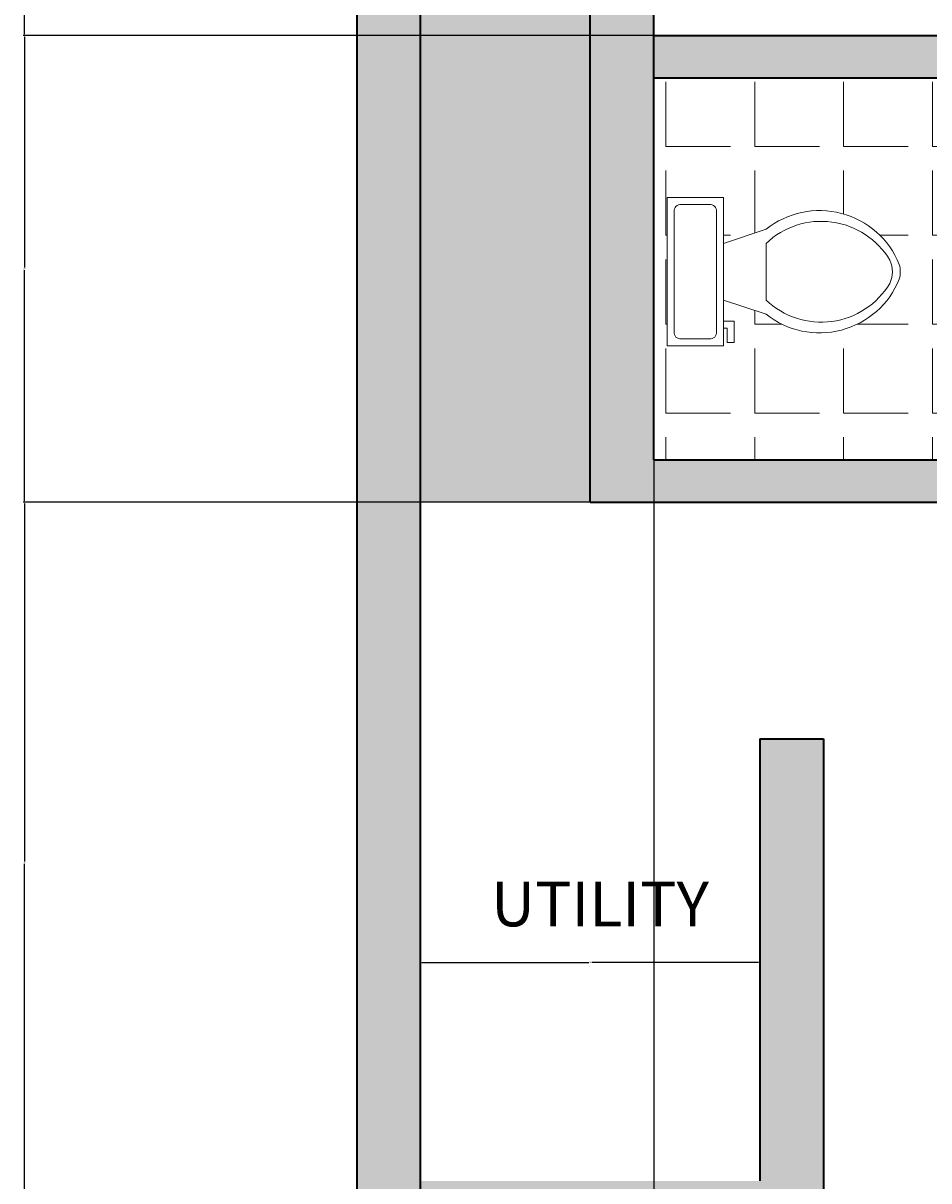
# Model space of a CAD drawing. Units: inches. Extents: x 2549 to 3108, y 1683 to 2362.
# Tile 6 of 30: x 2549 to 2678, y 1979 to 2142. Entities that reach past the tile are written whole.
import ezdxf

# ---------------------------------------------------------------- set-up
doc = ezdxf.new("R2010")
doc.units = ezdxf.units.IN
for name, color, linetype, lineweight in [('A-ANNO-DIMS', 2, 'Continuous', 18), ('A-AREA-IDEN', 7, 'Continuous', 18), ('A-FLOR', 7, 'Continuous', 25), ('A-FLOR-FIXT', 9, 'Continuous', 18), ('A-FLOR-PATT', 8, 'Continuous', 13), ('A-FURN-PATT', 9, 'Continuous', 13), ('A-WALL', 7, 'Continuous', 35), ('A-WALL-PATT', 89, 'Continuous', 13), ('C-PROP', 7, 'Continuous', 35)]:
    doc.layers.add(name, color=color, linetype=linetype, lineweight=lineweight)
for name, color, linetype, lineweight, true_color in [('C-PKNG-VEHI-PATT', 251, 'Continuous', 13, 0x636466), ('C-PROP-PATT', 252, 'Continuous', 13, 0x939598), ('C-PVMT-PATT', 9, 'Continuous', 13, 0xc7c8ca)]:
    doc.layers.add(name, color=color, linetype=linetype, lineweight=lineweight, true_color=true_color)
doc.styles.get("Standard").update_dxf_attribs({"font": 'arial.ttf'})
doc.dimstyles.get("Standard").update_dxf_attribs({"dimtxt": 0.18, "dimasz": 0.18, "dimexe": 0.18, "dimexo": 0.0625, "dimgap": 0.09, "dimtad": 0, "dimtih": 1, "dimtoh": 1, "dimdec": 4, "dimzin": 0, "dimdsep": 46, "dimtxsty": 'Standard', "dimcen": 0.09, "dimadec": 0, "dimazin": 0, "dimtfac": 1, "dimtdec": 4, "dimtofl": 0, "dimtmove": 0, "dimatfit": 3, "dimfxl": 1, "dimtolj": 1, "dimtzin": 0, "dimarcsym": 0})

# ---------------------------------------------------------------- blocks, each defined once
blk = doc.blocks.new('*U3')
for p, q in [((9.5, -6), (9.5, -2)), ((-8, -8.5), (-8, -8)), ((-7, -8), (-7, -9.5)), ((-4, -8), (-6, -14)), ((4, -8), (6, -14)), ((-10, -8.5), (-8, -8.5)), ((-10, -9.5), (-10, -8.5)), ((-7, -9.5), (-10, -9.5)), ((4, -14), (-4, -14))]:
    blk.add_line(p, q)
blk.add_lwpolyline([(10.5, -8), (10.5, 0), (-10.5, 0), (-10.5, -8)], close=True)
for points in [[(8.5, -1), (-8.5, -1)], [(-9.5, -2), (-9.5, -6)], [(-8.5, -7), (8.5, -7)]]:
    blk.add_lwpolyline(points)
for centre, radius, start, end in [((-8.62, -1.88), 0.884, 81.8699, 188.1301), ((8.62, -1.88), 0.884, 351.8699, 98.1301), ((-8.62, -6.12), 0.884, 171.8699, 278.1301), ((8.62, -6.12), 0.884, 261.8699, 8.1301), ((3.52, -21.58), 12.17, 141.4691, 247.9714), ((4.2, -21.82), 11.33, 136.3677, 238.9468), ((-3.52, -21.58), 12.17, 292.0284, 38.5307), ((-4.2, -21.82), 11.33, 301.053, 43.6321), ((0, -27.88), 4, 245.7318, 294.2682), ((0, -29), 4, 254.8605, 285.1395)]:
    blk.add_arc(centre, radius, start, end)
blk = doc.blocks.new('*D32')
at = {"layer": 'A-ANNO-DIMS', "color": 0, "lineweight": -2, "transparency": 16777216}
for p, q in [((2629.58, 2281.52), (2549.42, 2281.52)), ((2549.6, 2281.34), (2549.6, 2211.2)), ((2549.6, 2140.7), (2549.6, 2210.84)), ((2638.58, 2140.52), (2549.42, 2140.52))]:
    blk.add_line(p, q, dxfattribs=at)
at = {"layer": 'A-ANNO-DIMS', "color": 0, "transparency": 16777216}
for points in [[(2549.57, 2281.34), (2549.63, 2281.34), (2549.6, 2281.52)], [(2549.57, 2140.7), (2549.63, 2140.7), (2549.6, 2140.52)]]:
    blk.add_solid(points, dxfattribs=at)
at = {"layer": 'Defpoints', "color": 0, "transparency": 16777216}
for p in [(2549.6, 2281.52), (2629.64, 2281.52), (2638.64, 2140.52)]:
    blk.add_point(p, dxfattribs=at)
at = {"layer": 'A-ANNO-DIMS', "color": 0, "transparency": 16777216, "insert": (2549.6, 2211.02), "char_height": 0.18, "attachment_point": 5}
blk.add_mtext('\\A1;141', dxfattribs=at)
blk = doc.blocks.new('*D33')
at = {"layer": 'A-ANNO-DIMS', "color": 0, "lineweight": -2, "transparency": 16777216}
for p, q in [((2638.58, 2140.52), (2549.42, 2140.52)), ((2549.6, 2140.34), (2549.6, 2107.71)), ((2549.6, 2074.7), (2549.6, 2107.34)), ((2629.58, 2074.52), (2549.42, 2074.52))]:
    blk.add_line(p, q, dxfattribs=at)
at = {"layer": 'A-ANNO-DIMS', "color": 0, "transparency": 16777216}
for points in [[(2549.57, 2140.34), (2549.63, 2140.34), (2549.6, 2140.52)], [(2549.57, 2074.7), (2549.63, 2074.7), (2549.6, 2074.52)]]:
    blk.add_solid(points, dxfattribs=at)
at = {"layer": 'Defpoints', "color": 0, "transparency": 16777216}
for p in [(2549.6, 2140.52), (2638.64, 2140.52), (2629.64, 2074.52)]:
    blk.add_point(p, dxfattribs=at)
at = {"layer": 'A-ANNO-DIMS', "color": 0, "transparency": 16777216, "insert": (2549.6, 2107.52), "char_height": 0.18, "attachment_point": 5}
blk.add_mtext('\\A1;66', dxfattribs=at)
blk = doc.blocks.new('*D34')
at = {"layer": 'A-ANNO-DIMS', "color": 0, "lineweight": -2, "transparency": 16777216}
for p, q in [((2629.58, 2074.52), (2549.42, 2074.52)), ((2549.6, 2074.34), (2549.6, 2023.71)), ((2549.6, 1972.7), (2549.6, 2023.34)), ((2638.58, 1972.52), (2549.42, 1972.52))]:
    blk.add_line(p, q, dxfattribs=at)
at = {"layer": 'A-ANNO-DIMS', "color": 0, "transparency": 16777216}
for points in [[(2549.57, 2074.34), (2549.63, 2074.34), (2549.6, 2074.52)], [(2549.57, 1972.7), (2549.63, 1972.7), (2549.6, 1972.52)]]:
    blk.add_solid(points, dxfattribs=at)
at = {"layer": 'Defpoints', "color": 0, "transparency": 16777216}
for p in [(2549.6, 2074.52), (2629.64, 2074.52), (2638.64, 1972.52)]:
    blk.add_point(p, dxfattribs=at)
at = {"layer": 'A-ANNO-DIMS', "color": 0, "transparency": 16777216, "insert": (2549.6, 2023.52), "char_height": 0.18, "attachment_point": 5}
blk.add_mtext('\\A1;102', dxfattribs=at)
blk = doc.blocks.new('*D42')
at = {"layer": 'A-ANNO-DIMS', "color": 0, "lineweight": -2, "transparency": 16777216}
for p, q in [((2638.64, 2080.46), (2638.64, 1683.44)), ((2728.64, 2080.46), (2728.64, 1683.44)), ((2638.82, 1683.62), (2683.42, 1683.62)), ((2728.46, 1683.62), (2683.86, 1683.62))]:
    blk.add_line(p, q, dxfattribs=at)
at = {"layer": 'A-ANNO-DIMS', "color": 0, "transparency": 16777216}
for points in [[(2638.82, 1683.65), (2638.82, 1683.59), (2638.64, 1683.62)], [(2728.46, 1683.65), (2728.46, 1683.59), (2728.64, 1683.62)]]:
    blk.add_solid(points, dxfattribs=at)
at = {"layer": 'Defpoints', "color": 0, "transparency": 16777216}
for p in [(2638.64, 2080.52), (2728.64, 2080.52), (2728.64, 1683.62)]:
    blk.add_point(p, dxfattribs=at)
at = {"layer": 'A-ANNO-DIMS', "color": 0, "transparency": 16777216, "insert": (2683.64, 1683.62), "char_height": 0.18, "attachment_point": 5}
blk.add_mtext('\\A1;90', dxfattribs=at)
blk = doc.blocks.new('*D44')
at = {"layer": 'A-ANNO-DIMS', "color": 0, "lineweight": -2, "transparency": 16777216}
for p, q in [((2662.64, 2040.99), (2662.64, 1683.44)), ((2806.64, 2016.13), (2806.64, 1683.44)), ((2662.82, 1683.62), (2734.36, 1683.62)), ((2806.46, 1683.62), (2734.92, 1683.62))]:
    blk.add_line(p, q, dxfattribs=at)
at = {"layer": 'A-ANNO-DIMS', "color": 0, "transparency": 16777216}
for points in [[(2662.82, 1683.65), (2662.82, 1683.59), (2662.64, 1683.62)], [(2806.46, 1683.65), (2806.46, 1683.59), (2806.64, 1683.62)]]:
    blk.add_solid(points, dxfattribs=at)
at = {"layer": 'Defpoints', "color": 0, "transparency": 16777216}
for p in [(2662.64, 2041.06), (2806.64, 2016.19), (2806.64, 1683.62)]:
    blk.add_point(p, dxfattribs=at)
at = {"layer": 'A-ANNO-DIMS', "color": 0, "transparency": 16777216, "insert": (2734.64, 1683.62), "char_height": 0.18, "attachment_point": 5}
blk.add_mtext('\\A1;144', dxfattribs=at)
blk = doc.blocks.new('*D45')
at = {"layer": 'A-ANNO-DIMS', "color": 0, "lineweight": -2, "transparency": 16777216}
for p, q in [((2605.64, 1978.59), (2605.64, 2009.6)), ((2605.82, 2009.42), (2629.42, 2009.42)), ((2653.46, 2009.42), (2629.87, 2009.42)), ((2653.64, 1978.59), (2653.64, 2009.6))]:
    blk.add_line(p, q, dxfattribs=at)
at = {"layer": 'A-ANNO-DIMS', "color": 0, "transparency": 16777216}
for points in [[(2605.82, 2009.45), (2605.82, 2009.39), (2605.64, 2009.42)], [(2653.46, 2009.45), (2653.46, 2009.39), (2653.64, 2009.42)]]:
    blk.add_solid(points, dxfattribs=at)
at = {"layer": 'Defpoints', "color": 0, "transparency": 16777216}
for p in [(2653.64, 2009.42), (2605.64, 1978.52), (2653.64, 1978.52)]:
    blk.add_point(p, dxfattribs=at)
at = {"layer": 'A-ANNO-DIMS', "color": 0, "transparency": 16777216, "insert": (2629.64, 2009.42), "char_height": 0.18, "attachment_point": 5}
blk.add_mtext('\\A1;48', dxfattribs=at)

msp = doc.modelspace()

# ---------------------------------------------------------------- hatches: boundary and pattern name
at = {"layer": 'A-FLOR-PATT', "transparency": 33554567}
h = msp.add_hatch(dxfattribs=at)
h.set_pattern_fill('ANGLE', color=256, scale=1.8)
h.set_pattern_definition([(0, (0, 0), (0, 12.573), [9.144, -3.429]), (90, (0, 0), (-12.573, 8e-16), [9.144, -3.429])])
h.paths.add_polyline_path([(2806.6427, 2134.5237), (2785.7177, 2134.5237), (2747.213, 2134.5237), (2638.6427, 2134.5237), (2638.6427, 2080.5237), (2728.6427, 2080.5237), (2728.6427, 2109.4935), (2734.6427, 2109.4935), (2734.6427, 2080.5237), (2806.6427, 2080.5237)])
h.paths.add_polyline_path([(2673.3659, 2106.0669, -0.50131678), (2654.5049, 2101.1116), (2648.5048, 2103.1116), (2648.5048, 2100.1116), (2650.0048, 2100.1116), (2650.0048, 2097.1116), (2649.0048, 2097.1116), (2649.0048, 2099.1116), (2648.5048, 2099.1116), (2648.5048, 2096.6116), (2640.5048, 2096.6116), (2640.5048, 2117.6116), (2648.5048, 2117.6116), (2648.5048, 2111.1116), (2654.5047, 2113.1116, -0.50132349), (2673.3659, 2108.1563, -0.13289091)], flags=16)
h.paths.add_polyline_path([(2672.0278, 2105.4676, -0.48007965), (2654.5048, 2103.1117), (2654.5048, 2111.1116, -0.4800795), (2672.0278, 2108.7557, -0.21500378)], flags=0)
h.paths.add_polyline_path([(2647.5048, 2115.6116), (2647.5048, 2098.6116, -0.50000012), (2646.5048, 2097.6116), (2642.5048, 2097.6116, -0.50000012), (2641.5048, 2098.6116), (2641.5048, 2115.6116, -0.50000012), (2642.5048, 2116.6116), (2646.5048, 2116.6116, -0.50000012)], flags=0)
h.paths.add_polyline_path([(2748.8496, 2101.6383), (2798.148, 2101.6383), (2798.148, 2111.4248), (2748.8496, 2111.4248)], flags=24)
h.paths.add_polyline_path([(2685.2081, 2101.489), (2719.3253, 2101.489), (2719.3253, 2111.2819), (2685.2081, 2111.2819)], flags=24)
at = {"layer": 'A-FURN-PATT', "transparency": 33554567}
h = msp.add_hatch(color=256, dxfattribs=at)
h.dxf.hatch_style = 1
h.paths.add_polyline_path([(2708.7147, 2271.6737), (2675.2813, 2271.6737), (2675.2813, 2262.0404), (2708.7147, 2262.0404)])
h.paths.add_polyline_path([(2980.8246, 2271.6737), (2947.3913, 2271.6737), (2947.3913, 2262.0404), (2980.8246, 2262.0404)])
h.paths.add_polyline_path([(2748.8496, 2101.6383), (2798.148, 2101.6383), (2798.148, 2111.4248), (2748.8496, 2111.4248)], flags=9)
h.paths.add_polyline_path([(2685.2081, 2101.489), (2719.3253, 2101.489), (2719.3253, 2111.2819), (2685.2081, 2111.2819)], flags=9)
h.paths.add_polyline_path([(2814.6852, 1907.1328), (2847.8384, 1907.1328), (2847.8384, 1916.9258), (2814.6852, 1916.9258)], flags=9)
h.paths.add_polyline_path([(2814.3906, 1835.5864), (2848.0172, 1835.5864), (2848.0172, 1845.3794), (2814.3906, 1845.3794)], flags=9)
h.paths.add_polyline_path([(2800.5245, 1759.1674), (2853.7435, 1759.1674), (2853.7435, 1768.954), (2800.5245, 1768.954)], flags=9)
h.paths.add_polyline_path([(2972.4611, 1807.3305), (3015.3943, 1807.3305), (3015.3943, 1817.117), (2972.4611, 1817.117)], flags=9)
h.paths.add_polyline_path([(2902.3327, 1888.6731), (2937.9131, 1888.6731), (2937.9131, 1898.4661), (2902.3327, 1898.4661)], flags=9)
h.paths.add_polyline_path([(2712.1779, 1878.9039), (2754.1257, 1878.9039), (2754.1257, 1888.6904), (2712.1779, 1888.6904)], flags=9)
h.paths.add_polyline_path([(2614.0056, 2012.812), (2650.0251, 2012.812), (2650.0251, 2022.4371), (2614.0056, 2022.4371)], flags=9)
h.paths.add_polyline_path([(2713.3129, 2003.1645), (2747.4237, 2003.1645), (2747.4237, 2012.951), (2713.3129, 2012.951)], flags=9)
h.paths.add_polyline_path([(2950.1379, 2001.6934), (2982.2992, 2001.6934), (2982.2992, 2011.48), (2950.1379, 2011.48)], flags=9)
h.paths.add_polyline_path([(2940.864, 2238.5537), (2997.5066, 2238.5537), (2997.5066, 2248.3466), (2940.864, 2248.3466)], flags=9)
h.paths.add_polyline_path([(2821.5457, 2202.8348), (2855.663, 2202.8348), (2855.663, 2212.6278), (2821.5457, 2212.6278)], flags=9)
h.paths.add_polyline_path([(2661.8026, 2238.6249), (2718.4451, 2238.6249), (2718.4451, 2248.4179), (2661.8026, 2248.4179)], flags=9)
h = msp.add_hatch(color=256, dxfattribs=at)
h.dxf.hatch_style = 1
h.paths.add_polyline_path([(2906.5064, 1905.2148), (2905.2584, 1904.3827), (2907.0611, 1900.7772), (2908.3092, 1901.6092)])
h.paths.add_polyline_path([(2936.522, 1914.8044), (2935.2739, 1915.6364), (2932.6391, 1912.5856), (2933.8871, 1911.7535)])
h.paths.add_polyline_path([(2950.2508, 1905.6518), (2949.0027, 1906.4839), (2947.1999, 1902.8783), (2948.448, 1902.0463)])
h.paths.add_polyline_path([(2958.5713, 1918.1326), (2956.9072, 1919.242), (2952.4696, 1908.98, 1.38742744), (2954.9657, 1907.3159)])
h.paths.add_polyline_path([(2945.2585, 1927.0078), (2943.5944, 1928.1172), (2934.9965, 1920.6287, 1.38742744), (2937.4927, 1918.9646)])
h.paths.add_polyline_path([(2748.8496, 2101.6383), (2798.148, 2101.6383), (2798.148, 2111.4248), (2748.8496, 2111.4248)], flags=9)
h.paths.add_polyline_path([(2685.2081, 2101.489), (2719.3253, 2101.489), (2719.3253, 2111.2819), (2685.2081, 2111.2819)], flags=9)
h.paths.add_polyline_path([(2814.6852, 1907.1328), (2847.8384, 1907.1328), (2847.8384, 1916.9258), (2814.6852, 1916.9258)], flags=9)
h.paths.add_polyline_path([(2814.3906, 1835.5864), (2848.0172, 1835.5864), (2848.0172, 1845.3794), (2814.3906, 1845.3794)], flags=9)
h.paths.add_polyline_path([(2800.5245, 1759.1674), (2853.7435, 1759.1674), (2853.7435, 1768.954), (2800.5245, 1768.954)], flags=9)
h.paths.add_polyline_path([(2972.4611, 1807.3305), (3015.3943, 1807.3305), (3015.3943, 1817.117), (2972.4611, 1817.117)], flags=9)
h.paths.add_polyline_path([(2902.3327, 1888.6731), (2937.9131, 1888.6731), (2937.9131, 1898.4661), (2902.3327, 1898.4661)], flags=9)
h.paths.add_polyline_path([(2712.1779, 1878.9039), (2754.1257, 1878.9039), (2754.1257, 1888.6904), (2712.1779, 1888.6904)], flags=9)
h.paths.add_polyline_path([(2614.0056, 2012.812), (2650.0251, 2012.812), (2650.0251, 2022.4371), (2614.0056, 2022.4371)], flags=9)
h.paths.add_polyline_path([(2713.3129, 2003.1645), (2747.4237, 2003.1645), (2747.4237, 2012.951), (2713.3129, 2012.951)], flags=9)
h.paths.add_polyline_path([(2950.1379, 2001.6934), (2982.2992, 2001.6934), (2982.2992, 2011.48), (2950.1379, 2011.48)], flags=9)
h.paths.add_polyline_path([(2940.864, 2238.5537), (2997.5066, 2238.5537), (2997.5066, 2248.3466), (2940.864, 2248.3466)], flags=9)
h.paths.add_polyline_path([(2821.5457, 2202.8348), (2855.663, 2202.8348), (2855.663, 2212.6278), (2821.5457, 2212.6278)], flags=9)
h.paths.add_polyline_path([(2661.8026, 2238.6249), (2718.4451, 2238.6249), (2718.4451, 2248.4179), (2661.8026, 2248.4179)], flags=9)
at = {"layer": 'A-WALL-PATT'}
h = msp.add_hatch(color=256, dxfattribs=at)
h.dxf.hatch_style = 1
h.paths.add_polyline_path([(2638.6427, 2272.5237), (3034.6427, 2272.5237), (3034.6427, 1936.5237), (3043.6427, 1936.5237), (3043.6427, 2281.5237), (2629.6427, 2281.5237), (2629.6427, 2074.5237), (2812.6427, 2074.5237), (2812.6427, 2140.5237), (2785.7177, 2140.5237), (2785.7177, 2134.5237), (2806.6427, 2134.5237), (2806.6427, 2080.5237), (2638.6427, 2080.5237)])
h.paths.add_polyline_path([(2638.6427, 1972.5237), (2662.6427, 1972.5237), (2662.6427, 2041.0557), (2653.6427, 2041.0557), (2653.6427, 1978.5237), (2629.6427, 1978.5237), (2629.6427, 1795.5237), (2662.6427, 1795.5237), (2881.6427, 1795.5237), (2881.6427, 1936.5237), (2965.9351, 1936.5237), (2965.9351, 1974.5439), (2959.9351, 1974.5439), (2959.9351, 1945.5237), (2881.6427, 1945.5237), (2872.6427, 1945.5237), (2872.6427, 1804.5237), (2662.6427, 1804.5237), (2638.6427, 1804.5237)])
h = msp.add_hatch(color=256, dxfattribs=at)
h.dxf.hatch_style = 1
h.paths.add_polyline_path([(2747.213, 2140.5237), (2638.6427, 2140.5237), (2638.6427, 2134.5237), (2747.213, 2134.5237)])
h.paths.add_polyline_path([(2734.6427, 2109.4935), (2728.6427, 2109.4935), (2728.6427, 2080.5237), (2734.6427, 2080.5237)])
h.paths.add_polyline_path([(2812.6427, 2074.5237), (2806.6427, 2074.5237), (2806.6427, 2016.1911), (2812.6427, 2016.1911)])
h.paths.add_polyline_path([(2812.6427, 1945.5237), (2806.6427, 1945.5237), (2806.6427, 1885.5237), (2872.6427, 1885.5237), (2872.6427, 1891.5237), (2812.6427, 1891.5237)])
h.paths.add_polyline_path([(2812.6427, 1855.9859), (2806.6427, 1855.9859), (2806.6427, 1804.5237), (2812.6427, 1804.5237)])
at = {"layer": 'C-PKNG-VEHI-PATT'}
h = msp.add_hatch(color=256, dxfattribs=at)
h.dxf.hatch_style = 1
edge = h.paths.add_edge_path()
edge.add_ellipse((2935.7258, 1791.964), major_axis=(-50.66, 0), ratio=0.84230387, start_angle=248.165046, end_angle=265.722579)
edge.add_line((2938.911, 1834.5507), (2925.8653, 1834.5507))
edge.add_ellipse((2929.0505, 1791.964), major_axis=(50.66, 0), ratio=0.84230387, start_angle=94.277421, end_angle=111.834954)
edge.add_line((2912.8508, 1832.3947), (2914.2044, 1822.2495))
edge.add_ellipse((2930.6538, 1783.1023), major_axis=(-49.3014, 0), ratio=0.84230387, start_angle=-85.12993, end_angle=-67.208085, ccw=False)
edge.add_line((2927.1247, 1824.5225), (2937.6516, 1824.5225))
edge.add_ellipse((2934.1225, 1783.1023), major_axis=(49.3014, 0), ratio=0.84230387, start_angle=67.208085, end_angle=85.12993, ccw=False)
edge.add_line((2950.5719, 1822.2495), (2951.9255, 1832.3947))
edge = h.paths.add_edge_path()
edge.add_ellipse((2903.4793, 1857.3351), major_axis=(-34.7979, 0), ratio=0.84230387, start_angle=180, end_angle=209.43857)
edge.add_ellipse((2961.297, 1857.3351), major_axis=(34.7979, 0), ratio=0.84230387, start_angle=150.56143, end_angle=180)
edge.add_line((2926.4991, 1857.3351), (2926.4991, 1843.7609))
edge.add_ellipse((2924.1251, 1844.3143), major_axis=(-0.2209, 3.9278), ratio=0.60383358, start_angle=89.002014, end_angle=253.657408, ccw=False)
edge.add_line((2921.7512, 1844.2222), (2921.7512, 1853.3975))
edge.add_line((2921.7512, 1853.3975), (2925.269, 1855.8484))
edge.add_ellipse((2925.4782, 1855.4931), major_axis=(0.4584, 0), ratio=0.84230387, start_angle=90, end_angle=134.480211, ccw=False)
edge.add_line((2925.4782, 1855.8792), (2926.4991, 1855.8792))
edge.add_line((2926.4991, 1855.8792), (2926.4991, 1857.3351))
edge.add_ellipse((2961.297, 1857.3351), major_axis=(34.7979, 0), ratio=0.84230387, start_angle=150.56143, end_angle=180, ccw=False)
edge.add_line((2932.3882, 1873.6501), (2932.3882, 1875.7801))
edge.add_ellipse((2932.3882, 1875.3939), major_axis=(0.4584, 0), ratio=0.84230387, start_angle=90, end_angle=127.93313)
edge.add_line((2932.1366, 1875.7167), (2928.5915, 1873.7564))
edge.add_ellipse((2899.9271, 2002.4692), major_axis=(155.4756, 0), ratio=0.84230387, start_angle=-80.743434, end_angle=-77.445067, ccw=False)
edge.add_ellipse((2949.4402, 1715.2151), major_axis=(-189.1422, 0), ratio=0.84230387, start_angle=-79.790461, end_angle=-77.555373)
edge.add_ellipse((3300.3614, 1852.5642), major_axis=(-386.1662, 0), ratio=0.84230387, start_angle=-2.863715, end_angle=2.198541)
edge.add_ellipse((2929.0505, 1792.5159), major_axis=(-55.6192, 0), ratio=0.84230387, start_angle=-85.917589, end_angle=-72.280047, ccw=False)
edge.add_line((2925.7129, 1839.2798), (2939.0634, 1839.2798))
edge.add_ellipse((2935.7258, 1792.5159), major_axis=(55.6192, 0), ratio=0.84230387, start_angle=72.280047, end_angle=85.917589, ccw=False)
edge.add_ellipse((2564.4149, 1852.5642), major_axis=(-386.1662, 0), ratio=0.84230387, start_angle=177.801459, end_angle=182.863715)
edge.add_ellipse((2915.3361, 1715.2151), major_axis=(189.1422, 0), ratio=0.84230387, start_angle=77.555373, end_angle=79.790461)
edge.add_ellipse((2964.8492, 2002.4692), major_axis=(-155.4756, 0), ratio=0.84230387, start_angle=77.445067, end_angle=80.743434, ccw=False)
edge.add_line((2936.1848, 1873.7564), (2932.6397, 1875.7167))
edge.add_ellipse((2932.3882, 1875.3939), major_axis=(0.4584, 0), ratio=0.84230387, start_angle=52.06687, end_angle=90)
edge.add_line((2932.3882, 1875.7801), (2932.3882, 1873.6501))
edge.add_ellipse((2903.4793, 1857.3351), major_axis=(-34.7979, 0), ratio=0.84230387, start_angle=180, end_angle=209.43857, ccw=False)
edge.add_line((2938.2772, 1857.3351), (2938.2772, 1855.8792))
edge.add_line((2938.2772, 1855.8792), (2939.4059, 1855.8792))
edge.add_ellipse((2939.2981, 1855.4931), major_axis=(-0.4584, 0), ratio=0.84230387, start_angle=225.519789, end_angle=270, ccw=False)
edge.add_line((2939.5903, 1855.7906), (2943.0251, 1853.3975))
edge.add_line((2943.0251, 1853.3975), (2943.0251, 1844.2222))
edge.add_ellipse((2940.6512, 1844.3143), major_axis=(0.2209, 3.9278), ratio=0.60383358, start_angle=106.342592, end_angle=270.997986, ccw=False)
edge.add_line((2938.2772, 1843.7609), (2938.2772, 1857.3351))
edge = h.paths.add_edge_path()
edge.add_ellipse((2932.3882, 1865.1973), major_axis=(91.081, 0), ratio=0.84230387, start_angle=256.401865, end_angle=283.598135, ccw=False)
edge.add_line((2914.2044, 1790.0239), (2914.2044, 1778.3622))
edge.add_ellipse((2932.3882, 1853.5356), major_axis=(91.081, 0), ratio=0.84230387, start_angle=256.401865, end_angle=283.598135)
edge.add_line((2950.5719, 1778.3622), (2950.5719, 1790.0239))
edge = h.paths.add_edge_path()
edge.add_ellipse((2948.7383, 1772.3145), major_axis=(1.8336, 0), ratio=0.84230387, start_angle=0, end_angle=90)
edge.add_line((2948.7383, 1773.859), (2916.038, 1773.859))
edge.add_ellipse((2916.038, 1772.3145), major_axis=(1.8336, 0), ratio=0.84230387, start_angle=90, end_angle=180)
edge.add_line((2914.2044, 1772.3145), (2914.2044, 1760.2558))
edge.add_line((2914.2044, 1760.2558), (2950.5719, 1760.2558))
edge.add_line((2950.5719, 1760.2558), (2950.5719, 1772.3145))
h.paths.add_polyline_path([(2748.8496, 2101.6383), (2798.148, 2101.6383), (2798.148, 2111.4248), (2748.8496, 2111.4248)], flags=9)
h.paths.add_polyline_path([(2685.2081, 2101.489), (2719.3253, 2101.489), (2719.3253, 2111.2819), (2685.2081, 2111.2819)], flags=9)
h.paths.add_polyline_path([(2814.6852, 1907.1328), (2847.8384, 1907.1328), (2847.8384, 1916.9258), (2814.6852, 1916.9258)], flags=9)
h.paths.add_polyline_path([(2814.3906, 1835.5864), (2848.0172, 1835.5864), (2848.0172, 1845.3794), (2814.3906, 1845.3794)], flags=9)
h.paths.add_polyline_path([(2800.5245, 1759.1674), (2853.7435, 1759.1674), (2853.7435, 1768.954), (2800.5245, 1768.954)], flags=9)
h.paths.add_polyline_path([(2972.4611, 1807.3305), (3015.3943, 1807.3305), (3015.3943, 1817.117), (2972.4611, 1817.117)], flags=9)
h.paths.add_polyline_path([(2902.3327, 1888.6731), (2937.9131, 1888.6731), (2937.9131, 1898.4661), (2902.3327, 1898.4661)], flags=9)
h.paths.add_polyline_path([(2712.1779, 1878.9039), (2754.1257, 1878.9039), (2754.1257, 1888.6904), (2712.1779, 1888.6904)], flags=9)
h.paths.add_polyline_path([(2614.0056, 2012.812), (2650.0251, 2012.812), (2650.0251, 2022.4371), (2614.0056, 2022.4371)], flags=9)
h.paths.add_polyline_path([(2713.3129, 2003.1645), (2747.4237, 2003.1645), (2747.4237, 2012.951), (2713.3129, 2012.951)], flags=9)
h.paths.add_polyline_path([(2950.1379, 2001.6934), (2982.2992, 2001.6934), (2982.2992, 2011.48), (2950.1379, 2011.48)], flags=9)
h.paths.add_polyline_path([(2940.864, 2238.5537), (2997.5066, 2238.5537), (2997.5066, 2248.3466), (2940.864, 2248.3466)], flags=9)
h.paths.add_polyline_path([(2821.5457, 2202.8348), (2855.663, 2202.8348), (2855.663, 2212.6278), (2821.5457, 2212.6278)], flags=9)
h.paths.add_polyline_path([(2661.8026, 2238.6249), (2718.4451, 2238.6249), (2718.4451, 2248.4179), (2661.8026, 2248.4179)], flags=9)
at = {"layer": 'C-PROP-PATT'}
h = msp.add_hatch(color=256, dxfattribs=at)
h.dxf.hatch_style = 1
h.paths.add_polyline_path([(3076.6427, 2314.5237), (2596.6427, 2314.5237), (2596.6427, 1714.5237), (2881.84, 1714.5237), (2881.84, 1723.5237), (2605.6427, 1723.5237), (2605.6427, 2305.5237), (3067.6427, 2305.5237), (3067.6427, 1723.5237), (3067.6427, 1714.5237), (3076.6427, 1714.5237)])
at = {"layer": 'C-PVMT-PATT'}
h = msp.add_hatch(color=256, dxfattribs=at)
h.dxf.hatch_style = 1
h.paths.add_polyline_path([(3067.6427, 2305.5237), (2605.6427, 2305.5237), (2605.6427, 2074.5237), (2629.6427, 2074.5237), (2629.6427, 2281.5237), (3043.6427, 2281.5237), (3043.6427, 1885.5237), (3043.6427, 1872.8745), (3031.1672, 1872.8745), (3031.1672, 1862.5731), (2995.8054, 1862.5731), (2995.8054, 1872.8745), (2983.1752, 1872.8745), (2983.1752, 1885.5237), (2881.6427, 1885.5237), (2881.6427, 1795.5237), (2751.0977, 1795.5237), (2751.0977, 1761.5237), (2786.1577, 1761.5237), (2786.1577, 1723.5237), (2881.84, 1723.5237), (2881.84, 1714.5237), (3067.6427, 1714.5237), (3067.6427, 1723.5237)])
edge = h.paths.add_edge_path(flags=16)
edge.add_ellipse((2949.4402, 1710.9683), major_axis=(-194.1014, 0), ratio=0.84230387, start_angle=-77.874034, end_angle=-76.219471, ccw=False)
edge.add_ellipse((2949.4402, 1715.2151), major_axis=(-189.1422, 0), ratio=0.84230387, start_angle=-79.790461, end_angle=-77.555373, ccw=False)
edge.add_ellipse((2899.9271, 2002.4692), major_axis=(155.4756, 0), ratio=0.84230387, start_angle=-80.743434, end_angle=-77.445067)
edge.add_line((2928.5915, 1873.7564), (2932.3882, 1875.8558))
edge.add_line((2932.3882, 1875.8558), (2936.1848, 1873.7564))
edge.add_ellipse((2964.8492, 2002.4692), major_axis=(-155.4756, 0), ratio=0.84230387, start_angle=77.445067, end_angle=80.743434)
edge.add_ellipse((2915.3361, 1715.2151), major_axis=(189.1422, 0), ratio=0.84230387, start_angle=77.555373, end_angle=79.790461, ccw=False)
edge.add_ellipse((2915.3361, 1710.9683), major_axis=(-194.1014, 0), ratio=0.84230387, start_angle=256.219471, end_angle=257.874034, ccw=False)
edge.add_ellipse((2628.2871, 1850.2612), major_axis=(-327.2532, 0), ratio=0.84230387, start_angle=182.17995, end_angle=183.650428, ccw=False)
edge.add_ellipse((2955.5637, 1861.9334), major_axis=(-0.9168, 0), ratio=0.84230387, start_angle=180, end_angle=270, ccw=False)
edge.add_line((2956.4805, 1862.3857), (2956.4805, 1846.4866))
edge.add_ellipse((2955.5637, 1846.939), major_axis=(-0.9168, 0), ratio=0.84230387, start_angle=90, end_angle=180, ccw=False)
edge.add_ellipse((-3607.0606, 1835.832), major_axis=(-6562.6242, 0), ratio=0.84230387, start_angle=179.61613322, end_angle=180.09022909, ccw=False)
edge.add_ellipse((2955.5637, 1791.0926), major_axis=(0.9168, 0), ratio=0.84230387, start_angle=0, end_angle=90, ccw=False)
edge.add_line((2956.4805, 1791.545), (2956.4805, 1775.6459))
edge.add_ellipse((2955.5637, 1776.0982), major_axis=(0.9168, 0), ratio=0.84230387, start_angle=270, end_angle=360, ccw=False)
edge.add_ellipse((-3607.0606, 1835.832), major_axis=(-6562.6242, 0), ratio=0.84230387, start_angle=179.3813568, end_angle=179.47172853, ccw=False)
edge.add_ellipse((2954.5907, 1763.8768), major_axis=(-1.3752, 0), ratio=0.84230387, start_angle=179.371763, end_angle=248.464757, ccw=False)
edge.add_ellipse((-3607.519, 1835.832), major_axis=(-6564.0409, 0), ratio=0.842303863, start_angle=179.35344594, end_angle=179.37176282, ccw=False)
edge.add_ellipse((2952.6829, 1761.8002), major_axis=(3.2503, 0), ratio=0.84230387, start_angle=-90, end_angle=-0.646554, ccw=False)
edge.add_line((2952.6829, 1759.0625), (2912.0934, 1759.0625))
edge.add_ellipse((2912.0934, 1761.8002), major_axis=(3.2503, 0), ratio=0.84230387, start_angle=180.646554, end_angle=270, ccw=False)
edge.add_ellipse((9472.2953, 1835.832), major_axis=(-6564.0409, 0), ratio=0.842303871, start_angle=0.62823722, end_angle=0.6465541, ccw=False)
edge.add_ellipse((2910.1856, 1763.8768), major_axis=(1.3752, 0), ratio=0.84230387, start_angle=111.535244, end_angle=180.628237, ccw=False)
edge.add_ellipse((9471.8369, 1835.832), major_axis=(-6562.6242, 0), ratio=0.84230387, start_angle=0.52827147, end_angle=0.6465541, ccw=False)
edge.add_ellipse((2909.2126, 1776.0982), major_axis=(-0.9168, 0), ratio=0.84230387, start_angle=0, end_angle=90, ccw=False)
edge.add_line((2908.2958, 1775.6459), (2908.2958, 1791.545))
edge.add_ellipse((2909.2126, 1791.0926), major_axis=(-0.9168, 0), ratio=0.84230387, start_angle=-90, end_angle=0, ccw=False)
edge.add_ellipse((9471.8369, 1835.832), major_axis=(-6562.6242, 0), ratio=0.84230387, start_angle=-0.09022909, end_angle=0.38386678, ccw=False)
edge.add_ellipse((2909.2126, 1846.939), major_axis=(-0.9168, 0), ratio=0.84230387, start_angle=0, end_angle=90, ccw=False)
edge.add_line((2908.2958, 1846.4866), (2908.2958, 1862.3857))
edge.add_ellipse((2909.2126, 1861.9334), major_axis=(0.9168, 0), ratio=0.84230387, start_angle=90, end_angle=180, ccw=False)
edge.add_ellipse((3236.4892, 1850.2612), major_axis=(327.2532, 0), ratio=0.84230387, start_angle=176.349572, end_angle=177.82005, ccw=False)
edge = h.paths.add_edge_path(flags=0)
edge.add_ellipse((2903.4793, 1857.3351), major_axis=(-34.7979, 0), ratio=0.84230387, start_angle=180, end_angle=209.43857, ccw=False)
edge.add_line((2938.2772, 1857.3351), (2938.2772, 1855.8792))
edge.add_line((2938.2772, 1855.8792), (2939.4631, 1855.8792))
edge.add_line((2939.4631, 1855.8792), (2943.0251, 1853.3975))
edge.add_line((2943.0251, 1853.3975), (2943.0251, 1844.2222))
edge.add_ellipse((2940.6512, 1844.3143), major_axis=(0.2209, 3.9278), ratio=0.60383358, start_angle=106.342592, end_angle=270.997986, ccw=False)
edge.add_line((2938.2772, 1843.7609), (2938.2772, 1857.3351))
edge.add_ellipse((2903.4793, 1857.3351), major_axis=(-34.7979, 0), ratio=0.84230387, start_angle=180, end_angle=209.43857)
edge.add_ellipse((2961.297, 1857.3351), major_axis=(34.7979, 0), ratio=0.84230387, start_angle=150.56143, end_angle=180)
edge.add_line((2926.4991, 1857.3351), (2926.4991, 1843.7609))
edge.add_ellipse((2924.1251, 1844.3143), major_axis=(-0.2209, 3.9278), ratio=0.60383358, start_angle=89.002014, end_angle=253.657408, ccw=False)
edge.add_line((2921.7512, 1844.2222), (2921.7512, 1853.3975))
edge.add_line((2921.7512, 1853.3975), (2925.3132, 1855.8792))
edge.add_line((2925.3132, 1855.8792), (2926.4991, 1855.8792))
edge.add_line((2926.4991, 1855.8792), (2926.4991, 1857.3351))
edge.add_ellipse((2961.297, 1857.3351), major_axis=(34.7979, 0), ratio=0.84230387, start_angle=150.56143, end_angle=180, ccw=False)
edge = h.paths.add_edge_path(flags=0)
edge.add_ellipse((2929.0505, 1791.964), major_axis=(50.66, 0), ratio=0.84230387, start_angle=94.277421, end_angle=111.834954, ccw=False)
edge.add_line((2925.8653, 1834.5507), (2938.911, 1834.5507))
edge.add_ellipse((2935.7258, 1791.964), major_axis=(-50.66, 0), ratio=0.84230387, start_angle=248.165046, end_angle=265.722579, ccw=False)
edge.add_line((2951.9255, 1832.3947), (2950.5719, 1822.2495))
edge.add_ellipse((2934.1225, 1783.1023), major_axis=(49.3014, 0), ratio=0.84230387, start_angle=67.208085, end_angle=85.12993)
edge.add_line((2937.6516, 1824.5225), (2927.1247, 1824.5225))
edge.add_ellipse((2930.6538, 1783.1023), major_axis=(-49.3014, 0), ratio=0.84230387, start_angle=-85.12993, end_angle=-67.208085)
edge.add_line((2914.2044, 1822.2495), (2912.8508, 1832.3947))
edge = h.paths.add_edge_path(flags=0)
edge.add_line((2910.1338, 1829.4651), (2912.6432, 1821.2711))
edge.add_ellipse((5203.7787, 1816.4367), major_axis=(-2291.1426, 0), ratio=0.84230387, start_angle=-0.1208974, end_angle=0.3640763)
edge.add_line((2912.7012, 1801.8782), (2910.3305, 1792.5698))
edge.add_ellipse((9471.8369, 1835.832), major_axis=(-6561.7074, 0), ratio=0.84230387, start_angle=0.05559431, end_angle=0.37776419, ccw=False)
edge = h.paths.add_edge_path(flags=0)
edge.add_ellipse((-3607.0606, 1835.832), major_axis=(6561.7074, 0), ratio=0.84230387, start_angle=-0.37776419, end_angle=-0.05559431, ccw=False)
edge.add_line((2954.4458, 1792.5698), (2952.0751, 1801.8782))
edge.add_ellipse((660.9976, 1816.4367), major_axis=(2291.1426, 0), ratio=0.84230387, start_angle=-0.3640763, end_angle=0.1208974)
edge.add_line((2952.1331, 1821.2711), (2954.6425, 1829.4651))
edge = h.paths.add_edge_path(flags=0)
edge.add_ellipse((2932.3882, 1865.1973), major_axis=(91.081, 0), ratio=0.84230387, start_angle=256.401865, end_angle=283.598135)
edge.add_line((2950.5719, 1790.0239), (2950.5719, 1778.3622))
edge.add_ellipse((2932.3882, 1853.5356), major_axis=(91.081, 0), ratio=0.84230387, start_angle=256.401865, end_angle=283.598135, ccw=False)
edge.add_line((2914.2044, 1778.3622), (2914.2044, 1790.0239))
edge = h.paths.add_edge_path(flags=0)
edge.add_line((2916.038, 1773.859), (2948.7383, 1773.859))
edge.add_ellipse((2948.7383, 1772.3145), major_axis=(1.8336, 0), ratio=0.84230387, start_angle=0, end_angle=90, ccw=False)
edge.add_line((2950.5719, 1772.3145), (2950.5719, 1760.2558))
edge.add_line((2950.5719, 1760.2558), (2914.2044, 1760.2558))
edge.add_line((2914.2044, 1760.2558), (2914.2044, 1772.3145))
edge.add_ellipse((2916.038, 1772.3145), major_axis=(1.8336, 0), ratio=0.84230387, start_angle=90, end_angle=180, ccw=False)
h.paths.add_polyline_path([(2629.6427, 1978.5237), (2605.6427, 1978.5237), (2605.6427, 1723.5237), (2629.6427, 1723.5237), (2629.6427, 1795.5237)], flags=17)
h.paths.add_polyline_path([(2800.5245, 1759.1674), (2853.7435, 1759.1674), (2853.7435, 1768.954), (2800.5245, 1768.954)], flags=24)
h.paths.add_polyline_path([(2972.4611, 1807.3305), (3015.3943, 1807.3305), (3015.3943, 1817.117), (2972.4611, 1817.117)], flags=24)

# ---------------------------------------------------------------- linework, layer by layer
at = {"layer": 'A-FLOR'}
msp.add_line((2629.6427, 2074.5237), (2605.6427, 2074.5237), dxfattribs=at)
at = {"layer": 'A-WALL'}
for p, q in [((2629.6427, 2074.5237), (2629.6427, 2281.5237)), ((2638.6427, 2080.5237), (2638.6427, 2272.5237)), ((2638.6427, 2140.5237), (2747.213, 2140.5237)), ((2638.6427, 2134.5237), (2747.213, 2134.5237)), ((2638.6427, 2080.5237), (2806.6427, 2080.5237)), ((2629.6427, 2074.5237), (2812.6427, 2074.5237)), ((2653.6427, 2041.0557), (2653.6427, 1978.5237)), ((2653.6427, 2041.0557), (2662.6427, 2041.0557)), ((2662.6427, 2041.0557), (2662.6427, 1972.5237))]:
    msp.add_line(p, q, dxfattribs=at)
at = {"layer": 'C-PROP'}
msp.add_lwpolyline([(2596.6427, 2314.5237), (3076.6427, 2314.5237), (3076.6427, 1714.5237), (2596.6427, 1714.5237)], close=True, dxfattribs=at)
msp.add_lwpolyline([(2881.84, 1723.5237), (2605.6427, 1723.5237), (2605.6427, 2305.5237), (3067.6427, 2305.5237), (3067.6427, 1723.5237)], dxfattribs=at)

# ---------------------------------------------------------------- block references
at = {"layer": 'A-FLOR-FIXT', "rotation": 90}
msp.add_blockref('*U3', (2640.5048, 2107.1116), dxfattribs=at)

# ---------------------------------------------------------------- texts
at = {"layer": 'A-AREA-IDEN'}
msp.add_text('UTILITY', height=6.30916, dxfattribs=at).set_placement((2615.6098, 2014.5237))

# ---------------------------------------------------------------- dimensions: what is measured, and where the dimension line sits
at = {"layer": 'A-ANNO-DIMS'}
for base, p1, p2, angle, picture, middle in [((2549.6048, 2281.5237), (2638.6427, 2140.5237), (2629.6427, 2281.5237), 90, '*D32', (2549.6048, 2211.0237)), ((2549.6048, 2140.5237), (2629.6427, 2074.5237), (2638.6427, 2140.5237), 90, '*D33', (2549.6048, 2107.5237)), ((2549.6048, 2074.5237), (2638.6427, 1972.5237), (2629.6427, 2074.5237), 90, '*D34', (2549.6048, 2023.5237)), ((2653.6427, 2009.4237), (2605.6427, 1978.5237), (2653.6427, 1978.5237), 0, '*D45', (2629.6427, 2009.4237))]:
    dim = msp.add_linear_dim(base=base, p1=p1, p2=p2, angle=angle, dimstyle='Standard', override={"dimdec": 0, "dimlfac": 1, "dimrnd": 0, "dimzin": 0, "dimdsep": 46, "dimlunit": 2}, dxfattribs=at)
    dim.commit()
    dim.dimension.update_dxf_attribs({"geometry": picture, "text_midpoint": middle})
for base, p1, p2, picture, middle in [((2728.6427, 1683.6237), (2638.6427, 2080.5237), (2728.6427, 2080.5237), '*D42', (2683.6427, 1683.6237)), ((2806.6427, 1683.6237), (2662.6427, 2041.0557), (2806.6427, 2016.1911), '*D44', (2734.6427, 1683.6237))]:
    dim = msp.add_linear_dim(base=base, p1=p1, p2=p2, dimstyle='Standard', override={"dimdec": 0, "dimlfac": 1, "dimrnd": 0, "dimzin": 0, "dimdsep": 46, "dimlunit": 2}, dxfattribs=at)
    dim.commit()
    dim.dimension.update_dxf_attribs({"geometry": picture, "text_midpoint": middle})

doc.saveas('drawing.dxf')
